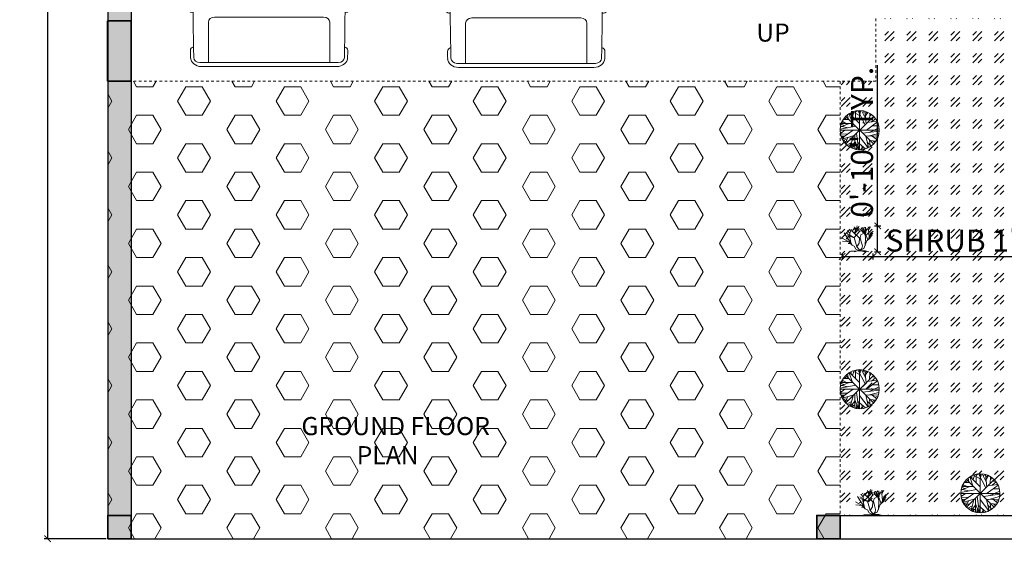
# Model space of a CAD drawing. Units: inches. Extents: x 3799 to 20199, y 1682 to 8087.
# Tile 6 of 30: x 10985 to 11366, y 2123 to 2325. Entities that reach past the tile are written whole.
import ezdxf

# ---------------------------------------------------------------- set-up
doc = ezdxf.new("R2010")
doc.units = ezdxf.units.IN
doc.linetypes.add('JIS_02_1.0', pattern=[2, 1, -1])
for name, color, linetype, lineweight in [('A-ANNO-DIMS', 2, 'Continuous', 18), ('A-ANNO-SYMB', 3, 'Continuous', 18), ('A-ANNO-TITL', 7, 'Continuous', 25), ('A-COLS', 251, 'Continuous', 35), ('A-SITE-OVHD', 8, 'JIS_02_1.0', 18), ('A-SITE-VEHC', 8, 'Continuous', 13), ('A-WALL-PATT', 252, 'Continuous', 13), ('C-PROP', 7, 'Continuous', 25), ('L-PAVE', 253, 'Continuous', 13), ('L-PLNT', 94, 'Continuous', 13), ('L-PLNT-PATT', 94, 'Continuous', 13)]:
    doc.layers.add(name, color=color, linetype=linetype, lineweight=lineweight)
doc.styles.get("Standard").update_dxf_attribs({"font": 'arial.ttf'})
doc.dimstyles.new('ISO-25', dxfattribs={"dimtxt": 8.5, "dimasz": 2.5, "dimexe": 1.25, "dimexo": 0.625, "dimtad": 1, "dimdec": 0, "dimlunit": 3, "dimtxsty": 'Standard', "dimblk": 'ARCHTICK', "dimcen": 2.5, "dimadec": 0, "dimazin": 0, "dimtfac": 1, "dimtdec": 0, "dimtmove": 0, "dimatfit": 3, "dimfxl": 1, "dimarcsym": 0})

# ---------------------------------------------------------------- blocks, each defined once
blk = doc.blocks.new('Shrub - elevation')
for p, q in [((-16.8, 16.32), (-18.72, 18.72)), ((-14.88, 18.24), (-17.76, 19.2)), ((-16.8, 16.32), (-15.36, 19.68)), ((-14.88, 18.24), (-12.96, 20.64)), ((-8.16, 12), (-14.88, 18.24)), ((-13.325, 16.724), (-11.433, 18.289)), ((-12.96, 12.48), (-8.16, 17.76)), ((-12.471, 19.775), (-12.898, 22.044)), ((-11.677, 19.071), (-12.471, 19.775)), ((-11.28, 19.619), (-12.104, 21.184)), ((-12.043, 15.628), (-11.921, 18.836)), ((-11.982, 16.802), (-10.579, 18.054)), ((-11.921, 18.836), (-10.64, 20.401)), ((-11.433, 18.289), (-10.457, 22.749)), ((-10.579, 18.054), (-9.846, 19.697)), ((-8.16, 17.76), (-10.56, 21.6)), ((-9.48, 19.775), (-8.992, 22.592)), ((-7.2, 19.68), (-8.64, 20.16)), ((-8.16, 17.76), (-5.28, 19.2)), ((-7.2, 19.68), (-6.24, 21.12)), ((-4.8, 16.32), (-7.2, 19.68)), ((-5.086, 17.741), (-5.513, 21.34)), ((-5.28, 19.2), (-3.84, 21.6)), ((-3.377, 15.315), (-5.086, 17.819)), ((-2.88, 12.96), (-4.32, 19.68)), ((-3.84, 16.8), (-0.96, 20.64)), ((-3.377, 18.602), (-2.888, 21.575)), ((-2.766, 16.802), (-3.377, 18.602)), ((-2.88, 15.84), (-2.4, 20.16)), ((-0.508, 21.888), (-0.081, 20.558)), ((-0.203, 19.149), (0.102, 21.34)), ((0.346, 13.203), (-0.203, 19.149)), ((-0.142, 19.384), (0.59, 20.401)), ((-0.02, 20.01), (0.896, 21.105)), ((0.041, 20.714), (1.384, 22.044)), ((0.102, 21.34), (0.835, 21.888)), ((1.323, 16.254), (3.642, 18.289)), ((-17.76, 8.64), (-23.663, 11.961)), ((-17.76, 8.64), (-23.128, 9.222)), ((-18.24, 11.04), (-21.755, 16.655)), ((-18.24, 11.04), (-20.16, 11.52)), ((-12.96, 12.48), (-19.68, 16.32)), ((-13.92, 12.48), (-19.2, 14.88)), ((-15.84, 8.16), (-18.24, 11.04)), ((-16.8, 12.48), (-17.76, 12.96)), ((-16.8, 12.48), (-16.8, 16.32)), ((-15.84, 8.16), (-16.8, 12.48)), ((-12.96, 12.48), (-13.92, 12.48)), ((-10.56, 4.32), (-12.96, 12.48)), ((-8.64, 7.68), (-8.16, 12)), ((-7.68, 12.48), (-7.2, 14.88)), ((-6.72, 8.64), (-7.68, 12.48)), ((-7.2, 14.88), (-3.84, 16.8)), ((-4.32, 2.88), (-1.92, 9.6)), ((-3.36, 5.28), (-2.88, 12.96)), ((-0.96, 10.56), (-2.88, 15.84)), ((-1.92, 9.6), (0.96, 12)), ((-0.48, 10.8), (0.346, 13.203)), ((0.346, 13.203), (1.323, 16.254)), ((0.96, 12), (1.44, 15.36)), ((0.96, 12), (2.88, 14.88)), ((1.44, 15.36), (2.88, 17.28)), ((1.92, 13.44), (2.4, 15.36)), ((2.4, 15.36), (3.36, 16.32)), ((-16.32, 7.2), (-18.24, 7.2)), ((-14.88, 5.76), (-17.76, 8.64)), ((-15.84, 0.48), (-17.76, 0)), ((-14.88, 5.76), (-15.84, 8.16)), ((-13.44, 0.48), (-15.84, 0.48)), ((-12.96, 4.8), (-14.88, 5.76)), ((-9.6, 0.96), (-13.44, 0.48)), ((-11.52, 2.4), (-12.96, 4.8)), ((-9.6, 0.96), (-12.96, 0)), ((-8.64, 0.96), (-11.52, 2.4)), ((-10.56, 4.32), (-8.64, 7.68)), ((-8.64, 1.92), (-10.56, 4.32)), ((-9.6, 0.96), (-7.68, 0.96)), ((-8.64, 0.96), (-4.32, 2.88)), ((-8.64, 0.96), (-6.24, 2.88)), ((-8.64, 0.96), (-8.64, 1.92)), ((-8.64, 0.96), (-2.88, 0.96)), ((-7.68, 0.96), (-6.24, 0.48)), ((-5.76, 5.28), (-6.72, 8.64)), ((-6.24, 2.88), (-5.76, 5.28)), ((-6.24, 0.48), (-3.36, 0)), ((-2.88, 0.96), (0, 0))]:
    blk.add_line(p, q)
blk = doc.blocks.new('Tree - deciduous plan')
for p, q in [((-49.8627, 32.8214), (-32.7853, 32.8214)), ((-45.8134, 38.2383), (-40.5318, 33.0471)), ((-43.8768, 36.4326), (-44.405, 40.2696)), ((42, 42), (-42, -42)), ((42, -42), (-42, 42)), ((-40.1797, 44.558), (-36.4825, 43.2038)), ((-37.0107, 47.0408), (-35.25, 35.5298)), ((-32.6092, 50.4264), (-23.2782, 23.5674)), ((-31.2008, 51.1035), (-0.2149, 20.1818)), ((-26.4472, 46.5894), (-26.2712, 53.8116)), ((-22.0458, 42.0753), (-16.5881, 57.6486)), ((-21.1656, 55.8436), (-0.0388, 45.0094)), ((-12.5388, 54.9406), (-7.9613, 59.4546)), ((-12.3627, 32.1443), (-12.5388, 58.7776)), ((-5.3205, 59.6806), (16.5105, 16.7963)), ((2.426, 54.9406), (-1.4472, 59.9056)), ((0, 59.9996), (0, -60)), ((0.4894, 48.6208), (3.6584, 59.6806)), ((18.2711, 35.5298), (5.419, 59.6806)), ((9.8203, 51.5549), (12.8133, 58.5516)), ((19.6795, 19.5047), (16.3344, 57.6486)), ((17.0387, 51.1035), (23.2006, 55.1666)), ((17.7429, 43.6552), (25.4894, 54.2636)), ((31.6513, 50.8778), (30.2429, 30.5643)), ((31.1232, 42.5267), (35.8767, 48.1693)), ((36.2288, 25.1474), (48.9049, 35.0784)), ((37.1091, 37.1098), (46.6161, 37.5612)), ((-59.7219, 2.8025), (-12.0106, 12.0565)), ((-32.2571, 20.6333), (-59.1937, 9.348)), ((-58.6656, 12.7336), (-35.9543, 7.5424)), ((-57.081, 17.9248), (-47.0458, 14.7649)), ((-56.0247, 20.859), (-20.8134, 20.859)), ((-54.7923, 24.4702), (-47.75, 21.0847)), ((-54.6162, -24.7335), (-20.2853, 0.0941)), ((-53.2078, 27.4044), (-40.1797, 20.859)), ((54.3626, 25.3731), (20.9119, 0.3198)), ((23.3767, 23.3417), (53.3063, 27.4044)), ((29.3626, -6.6771), (59.4682, 7.091)), ((38.5175, 13.4107), (58.2359, 13.6364)), ((-60, 0), (60, 0)), ((-59.7219, -4.8714), (-54.2641, -6.6771)), ((-45.2853, -0.1316), (-59.0177, -10.0627)), ((-58.4895, -12.3197), (-36.4825, -11.6426)), ((-57.081, -18.4138), (-45.2853, -17.9624)), ((-52.6797, -18.188), (-55.4966, -22.0251)), ((-53.2078, -27.442), (-16.7641, -16.6081)), ((-38.9472, -29.0219), (-51.4472, -30.6018)), ((-47.2219, -19.3166), (-50.2148, -26.3135)), ((-46.5177, -30.1504), (-49.5106, -33.536)), ((-35.9543, -22.4765), (-44.0529, -40.5329)), ((-19.9331, -20.2194), (-28.5599, -52.721)), ((-14.8275, -15.0282), (-14.6515, -57.6865)), ((-10.074, -10.0627), (-2.5036, -59.7178)), ((-0.0388, -19.0909), (25.8415, -53.8495)), ((9.2922, -9.1598), (59.6443, -2.8401)), ((18.6232, -18.6394), (26.7218, -53.3981)), ((18.7992, -18.6394), (57.3556, -17.2853)), ((26.3697, -18.4138), (58.9401, -9.8369)), ((30.419, -30.1504), (32.3556, -50.0125)), ((38.1654, -18.188), (52.426, -29.0219)), ((45.9119, -24.0564), (55.595, -22.2508)), ((-32.4331, -32.4075), (-48.1021, -35.5674)), ((-43.7008, -34.6645), (-46.6937, -37.373)), ((-24.6867, -37.8244), (-38.7712, -45.7241)), ((-26.2712, -43.9185), (-34.7219, -48.6583)), ((-14.6515, -36.2445), (-27.6797, -52.9467)), ((-14.6515, -47.3041), (-25.0388, -54.3009)), ((-21.5177, -45.4984), (-19.9331, -56.1065)), ((-14.6515, -32.1818), (-3.912, -59.4922)), ((-8.4895, -47.5298), (-11.4825, -58.5893)), ((-6.3768, -52.721), (-9.3698, -58.815)), ((-6.2008, -36.2445), (17.919, -57.0094)), ((8.4119, -53.1724), (3.8344, -59.4922)), ((5.9471, -46.6269), (10.5246, -58.5893)), ((22.8485, -36.4702), (35.3485, -48.4326)), ((24.7852, -44.8213), (23.0246, -54.978)), ((31.4753, -31.279), (49.6091, -33.3103)), ((41.5105, -32.6332), (46.088, -38.0501))]:
    blk.add_line(p, q)
blk.add_circle((0, 0), 60)
blk = doc.blocks.new('_ArchTick')
at = {"color": 0, "linetype": 'ByBlock', "const_width": 0.15}
blk.add_lwpolyline([(-0.5, -0.5), (0.5, 0.5)], dxfattribs=at)
blk = doc.blocks.new('*D77')
at = {"layer": 'A-ANNO-DIMS', "color": 0, "lineweight": -2, "transparency": 16777216}
for p, q in [((11018.23, 3204.07), (10994.27, 3204.07)), ((10995.52, 3204.07), (10995.52, 2124.07)), ((11018.23, 2124.07), (10994.27, 2124.07))]:
    blk.add_line(p, q, dxfattribs=at)
at = {"layer": 'Defpoints', "color": 0, "transparency": 16777216}
for p in [(11018.85, 3204.07), (10995.52, 2124.07), (11018.85, 2124.07)]:
    blk.add_point(p, dxfattribs=at)
at = {"layer": 'A-ANNO-DIMS', "color": 0, "lineweight": -2, "transparency": 16777216, "xscale": 2.5, "yscale": 2.5, "zscale": 2.5}
for p, rotation in [((10995.52, 3204.07), 90), ((10995.52, 2124.07), 270)]:
    blk.add_blockref('_ArchTick', p, dxfattribs=dict(at, rotation=rotation))
at = {"layer": 'A-ANNO-DIMS', "color": 0, "transparency": 16777216, "insert": (10990.56, 2664.07), "char_height": 8.5, "attachment_point": 5, "rotation": 90}
blk.add_mtext("90'", dxfattribs=at)
blk = doc.blocks.new('*U92')
for p, q in [((46.55, 38.89), (22.35, 38.89)), ((136.7, 38.89), (160.9, 38.89)), ((21.1, 37.41), (21.1, 36.83)), ((47.8, 37.39), (47.8, 37.41)), ((87.99, 31.87), (74.76, 35.92)), ((134.31, 35.6), (119.29, 31.78)), ((135.45, 37.07), (135.45, 37.41)), ((162.15, 37.41), (162.15, 36.77)), ((186.47, -33.5), (186.47, 33.5)), ((70.03, 31.54), (86.41, 29.35)), ((138.42, 29.35), (157.25, 29.35)), ((186.47, 29.35), (167.01, 29.35)), ((188.4, -32.76), (188.4, 32.76)), ((164.52, 26.39), (164.52, -26.39)), ((32.27, 11.63), (36.13, 17.17)), ((36.13, 17.17), (50.94, 17.17)), ((32.12, 9.51), (32.12, 11.15)), ((58.92, -10.77), (58.92, 10.77)), ((66.55, -10.53), (66.55, 10.53)), ((186.47, -10.53), (186.47, 10.53)), ((3.27, 6.13), (0.1, 0.41)), ((29.77, 9.51), (51.68, 9.51)), ((82.74, 8.5), (82.74, -8.5)), ((0, 0), (51.68, 0)), ((0.1, -0.41), (3.27, -6.13)), ((29.77, -9.51), (51.68, -9.51)), ((32.12, -9.51), (32.12, -11.15)), ((32.27, -11.63), (36.13, -17.17)), ((36.13, -17.17), (50.94, -17.17)), ((86.41, -29.35), (70.03, -31.54)), ((87.99, -31.87), (74.76, -35.92)), ((134.31, -35.6), (119.29, -31.78)), ((157.25, -29.35), (138.42, -29.35)), ((167.01, -29.35), (186.47, -29.35)), ((21.1, -37.41), (21.1, -36.83)), ((47.8, -37.39), (47.8, -37.41)), ((135.45, -37.07), (135.45, -37.41)), ((162.15, -37.41), (162.15, -36.77)), ((46.55, -38.89), (22.35, -38.89)), ((136.7, -38.89), (160.9, -38.89))]:
    blk.add_line(p, q)
for centre, major_axis, ratio, start_param, end_param in [((22.35, 37.41), (0, -1.48), 0.842304, 3.141593, 4.712389), ((46.55, 37.41), (0, 1.48), 0.842304, -1.570796, 0), ((136.7, 37.41), (0, -1.48), 0.842304, 3.141593, 4.712389), ((160.9, 37.41), (0, 1.48), 0.842304, -1.570796, 0), ((266.03, -27.52), (0, 313.31), 0.842304, 1.367076, 1.39176), ((41.19, -490.86), (0, 528.23), 0.842304, 0.00281, 0.075598), ((64.48, -10555.62), (0, 10593.03), 0.842304, -0.013397, 0.002797), ((64.48, -10555.62), (0, -10591.55), 0.842304, 3.133765, 3.140441), ((180.63, 35.84), (0, 2.22), 0.842304, -0.013017, 1.249894), ((64.48, -10556.36), (0, 10595.31), 0.842304, -0.013397, -0.013017), ((183.98, 33.5), (0, -2.96), 0.842304, 1.570796, 3.128196), ((183.98, 32.76), (0, -5.25), 0.842304, 1.570796, 3.128196), ((37.47, -593.96), (0, -623.33), 0.842304, 3.096046, 3.200911), ((134.4, 5.39), (0, -89.78), 0.842304, 4.449482, 4.652344), ((135.29, 5.39), (0, 81.77), 0.842304, 1.245306, 1.50788), ((149.6, 2.8), (0, -79.58), 0.842304, 4.372215, 4.640744), ((95.79, -3666.35), (0, -3698.24), 0.842304, 3.134049, 3.144098), ((17.08, 0), (0, 147.02), 0.842304, 4.511394, 4.913384), ((35.91, 0), (0, 147.02), 0.842304, 4.511394, 4.913384), ((167.01, 26.39), (0, 2.96), 0.842304, 0, 1.570796), ((259.18, -27.52), (0, -305.3), 0.842304, 4.528606, 4.561838), ((-204.49, 52.4), (0, -250.96), 0.842304, 1.385369, 1.434372), ((13.04, 17.01), (0, 27.42), 0.842304, 4.435146, 4.718221), ((14.2, 17.01), (0, 27.42), 0.842304, 4.435146, 4.718221), ((50.79, 13.34), (6.34, -0.36), 0.603834, -1.395552, 1.581315), ((32.75, 11.15), (0, 0.74), 0.842304, 0.879714, 1.570796), ((29.77, -46.66), (0, 56.17), 0.842304, 0, 0.590319), ((0.62, 0), (0, -0.74), 0.842304, 4.131459, 5.293319), ((29.77, 46.66), (0, 56.17), 0.842304, 2.551274, 3.141593), ((-204.49, -52.4), (0, 250.96), 0.842304, -1.434372, -1.385369), ((13.04, -17.01), (0, -27.42), 0.842304, 1.564964, 1.848039), ((14.2, -17.01), (0, -27.42), 0.842304, 1.564964, 1.848039), ((149.6, -2.8), (0, -79.58), 0.842304, -1.499151, -1.230623), ((32.75, -11.15), (0, -0.74), 0.842304, 4.712389, 5.403472), ((134.4, -5.39), (0, -89.78), 0.842304, -1.510751, -1.307889), ((135.29, -5.39), (0, -81.77), 0.842304, -1.50788, -1.245306), ((259.18, 27.52), (0, 305.3), 0.842304, 1.721348, 1.754579), ((266.03, 27.52), (0, 313.31), 0.842304, 1.749832, 1.774517), ((37.47, 593.96), (0, -623.33), 0.842304, -0.059319, 0.045547), ((167.01, -26.39), (0, -2.96), 0.842304, 4.712389, 6.283185), ((95.79, 3666.35), (0, -3698.24), 0.842304, -0.002505, 0.007544), ((183.98, -32.76), (0, -5.25), 0.842304, 0.013397, 1.570796), ((41.19, 490.86), (0, -528.23), 0.842304, -0.075598, -0.00281), ((22.35, -37.41), (0, 1.48), 0.842304, 1.570796, 3.141593), ((64.48, 10555.62), (0, 10593.03), 0.842304, 3.138796, 3.15499), ((46.55, -37.41), (0, -1.48), 0.842304, 0, 1.570796), ((64.48, 10555.62), (0, -10591.55), 0.842304, 0.001152, 0.007828), ((136.7, -37.41), (0, -1.48), 0.842304, -1.570796, 0), ((160.9, -37.41), (0, 1.48), 0.842304, 3.141593, 4.712389), ((180.63, -35.84), (0, -2.22), 0.842304, -1.249894, 0.013017), ((64.48, 10556.36), (0, 10595.31), 0.842304, 3.15461, 3.15499), ((183.98, -33.5), (0, 2.96), 0.842304, 3.15499, 4.712389)]:
    blk.add_ellipse(centre, major_axis=major_axis, ratio=ratio, start_param=start_param, end_param=end_param)
at = {"extrusion": (0, 0, -1)}
blk.add_ellipse((50.79, -13.34), major_axis=(6.34, 0.36), ratio=0.603834, start_param=-1.395552, end_param=1.581315, dxfattribs=at)
blk = doc.blocks.new('*D300')
at = {"layer": 'A-ANNO-DIMS', "color": 0, "lineweight": -2, "transparency": 16777216}
for p, q in [((11302.78, 2234.32), (11302.78, 2231.9)), ((11302.78, 2233.15), (11314.75, 2233.15)), ((11314.75, 2234.32), (11314.75, 2231.9)), ((11314.75, 2233.15), (11415.14, 2233.15))]:
    blk.add_line(p, q, dxfattribs=at)
at = {"layer": 'Defpoints', "color": 0, "transparency": 16777216}
for p in [(11302.78, 2234.95), (11314.75, 2234.95), (11314.75, 2233.15)]:
    blk.add_point(p, dxfattribs=at)
at = {"layer": 'A-ANNO-DIMS', "color": 0, "lineweight": -2, "transparency": 16777216, "xscale": 2.5, "yscale": 2.5, "zscale": 2.5, "rotation": 180}
blk.add_blockref('_ArchTick', (11302.78, 2233.15), dxfattribs=at)
at = {"layer": 'A-ANNO-DIMS', "color": 0, "lineweight": -2, "transparency": 16777216, "xscale": 2.5, "yscale": 2.5, "zscale": 2.5}
blk.add_blockref('_ArchTick', (11314.75, 2233.15), dxfattribs=at)
at = {"layer": 'A-ANNO-DIMS', "color": 0, "transparency": 16777216, "insert": (11366.2, 2238.17), "char_height": 8.5, "attachment_point": 5}
blk.add_mtext('SHRUB 1\'-0" TYP.', dxfattribs=at)
blk = doc.blocks.new('*D301')
at = {"layer": 'A-ANNO-DIMS', "color": 0, "lineweight": -2, "transparency": 16777216}
for p, q in [((11316.55, 2244.93), (11316.55, 2307.09)), ((11315.38, 2244.93), (11317.8, 2244.93)), ((11316.55, 2234.95), (11316.55, 2244.93)), ((11315.38, 2234.95), (11317.8, 2234.95))]:
    blk.add_line(p, q, dxfattribs=at)
at = {"layer": 'Defpoints', "color": 0, "transparency": 16777216}
for p in [(11314.75, 2244.93), (11316.55, 2244.93), (11314.75, 2234.95)]:
    blk.add_point(p, dxfattribs=at)
at = {"layer": 'A-ANNO-DIMS', "color": 0, "lineweight": -2, "transparency": 16777216, "xscale": 2.5, "yscale": 2.5, "zscale": 2.5}
for p, rotation in [((11316.55, 2244.93), 90), ((11316.55, 2234.95), 270)]:
    blk.add_blockref('_ArchTick', p, dxfattribs=dict(at, rotation=rotation))
at = {"layer": 'A-ANNO-DIMS', "color": 0, "transparency": 16777216, "insert": (11311.58, 2277.26), "char_height": 8.5, "attachment_point": 5, "rotation": 90}
blk.add_mtext('0\'-10" TYP.', dxfattribs=at)

msp = doc.modelspace()

# ---------------------------------------------------------------- hatches: boundary and pattern name
at = {"layer": 'A-COLS'}
h = msp.add_hatch(color=256, dxfattribs=at)
h.dxf.hatch_style = 1
h.set_gradient(color1=(0, 0, 255), color2=(122, 175, 223))
h.paths.add_polyline_path([(11302.02, 2133.07), (11293.02, 2133.07), (11293.02, 2124.07), (11302.02, 2124.07)])
h.paths.add_polyline_path([(11027.85, 2133.07), (11018.85, 2133.07), (11018.85, 2124.07), (11027.85, 2124.07)])
h.paths.add_polyline_path([(11027.85, 2324.17), (11018.85, 2324.17), (11018.85, 2300.82), (11027.85, 2300.82)])
h.paths.add_polyline_path([(11027.85, 2493.31), (11018.85, 2493.31), (11018.85, 2469.95), (11027.85, 2469.95)])
at = {"layer": 'A-WALL-PATT'}
h = msp.add_hatch(color=256, dxfattribs=at)
h.dxf.hatch_style = 1
h.paths.add_polyline_path([(11027.85, 2469.95), (11018.85, 2469.95), (11018.85, 2324.17), (11027.85, 2324.17)])
h.paths.add_polyline_path([(11027.85, 2300.82), (11018.85, 2300.82), (11018.85, 2133.07), (11027.85, 2133.07)])
at = {"layer": 'L-PAVE'}
h = msp.add_hatch(dxfattribs=at)
h.set_pattern_fill('HEX', color=256, scale=2)
h.paths.add_polyline_path([(11302.02, 2300.82), (11018.85, 2300.82), (11018.85, 2124.07), (11302.02, 2124.07)])
h.paths.add_polyline_path([(11091.95, 2151.09), (11148.17, 2151.09), (11148.17, 2161.6), (11091.95, 2161.6)], flags=24)
h.paths.add_polyline_path([(11091.89, 2162.16), (11175.38, 2162.16), (11175.38, 2173.03), (11091.89, 2173.02)], flags=24)
at = {"layer": 'L-PLNT-PATT'}
h = msp.add_hatch(dxfattribs=at)
h.set_pattern_fill('GOST_GLASS', color=256)
h.paths.add_polyline_path([(11609.85, 2325.07), (11549.85, 2325.07), (11315.85, 2325.07), (11315.85, 2300.82), (11302.02, 2300.82), (11302.02, 2133.07), (11609.85, 2133.07)])
h.paths.add_polyline_path([(11496.55, 2144.31), (11496.62, 2144.39), (11496.58, 2144.52)], flags=16)
h.paths.add_polyline_path([(11491.91, 2145.12), (11493.01, 2143.36), (11494.28, 2143.99), (11494.28, 2144.01), (11494.36, 2143.39), (11494.73, 2142.84), (11494.91, 2142.94), (11495.46, 2143.67), (11495.33, 2142.52), (11496.19, 2140.15), (11495.75, 2139.78), (11494.7, 2136.83), (11492.98, 2136.07), (11493.22, 2135.99), (11492.8, 2135.99), (11491.54, 2136.62), (11490.91, 2137.68), (11490.07, 2138.1), (11489.64, 2139.15), (11489.22, 2141.04), (11489.22, 2142.73), (11489.64, 2143.71), (11490.07, 2143.57), (11491.02, 2144.77), (11491.12, 2144.24), (11491.46, 2143.95), (11491.73, 2144.28)], flags=16)
h.paths.add_polyline_path([(11491.31, 2142.42), (11493.01, 2140.83), (11492.8, 2138.94), (11491.96, 2137.47), (11490.91, 2141.04), (11491.77, 2141.99), (11490.77, 2142.92), (11491.35, 2143.4)], flags=0)
h.paths.add_polyline_path([(11455.55, 2140.87), (11453.52, 2140.87), (11451.69, 2140.04), (11455.54, 2140.52, 0.011687)], flags=16)
h.paths.add_polyline_path([(11451.82, 2137.03), (11451.82, 2136.94), (11451.92, 2136.93)], flags=16)
h.paths.add_polyline_path([(11447.97, 2140.87), (11447.97, 2135.62), (11447.21, 2136.28), (11446.7, 2139.6), (11446.1, 2139), (11446.11, 2136.84), (11446.26, 2136.47), (11446.11, 2136.28), (11446.12, 2134.9), (11445.36, 2134.39), (11445.25, 2135.18), (11446.11, 2136.28), (11446.1, 2138.85), (11445.88, 2138.78), (11443.88, 2136.78), (11442.77, 2136.56), (11443.44, 2138.06), (11441.62, 2137.52), (11442.08, 2138.6), (11442.26, 2138.61), (11442, 2138.42), (11441.62, 2137.52), (11445.88, 2138.78), (11447.97, 2140.87), (11447.97, 2143.39), (11445.18, 2146.18), (11445.72, 2147.71), (11447.97, 2146.55), (11447.97, 2148.2), (11448.27, 2147.82), (11448.02, 2146.98), (11450.07, 2142.97)], flags=16)
h.paths.add_polyline_path([(11551.41, 2140.65, -1), (11536.26, 2140.65, -1)])
h.paths.add_polyline_path([(11547.68, 2136.8), (11547.69, 2136.71), (11547.78, 2136.7)], flags=16)
h.paths.add_polyline_path([(11541.05, 2145.95), (11541.58, 2147.48), (11542.26, 2147.14), (11542.27, 2144.73)], flags=16)
h.paths.add_polyline_path([(11541.96, 2138.78), (11541.97, 2136.62), (11542.12, 2136.24), (11541.97, 2136.06), (11541.98, 2134.67), (11541.23, 2134.17), (11541.11, 2134.95), (11541.97, 2136.06), (11541.96, 2138.62), (11541.74, 2138.56), (11539.74, 2136.56), (11538.63, 2136.33), (11539.3, 2137.83), (11537.48, 2137.29), (11537.94, 2138.37), (11538.12, 2138.38), (11541.25, 2140.65), (11543.83, 2140.65)], flags=16)
h.paths.add_polyline_path([(11584.29, 2268.01), (11584.1, 2268.75), (11584.25, 2269.39), (11584.02, 2270.08), (11583.56, 2270.33), (11584.06, 2270.63), (11584.18, 2271.22), (11584.1, 2271.81), (11584.48, 2272.21), (11584.83, 2272.85), (11584.45, 2273.49), (11583.87, 2273.79), (11584.72, 2273.79), (11585.41, 2273.89), (11585.79, 2274.33), (11585.79, 2274.73), (11586.3, 2275.17), (11587.03, 2275.22), (11587.76, 2275.66), (11588.26, 2275.62), (11588.72, 2275.91), (11589.22, 2275.66), (11589.53, 2276.8), (11589.69, 2275.91), (11590.23, 2275.81), (11590.92, 2276.11), (11591.46, 2276.26), (11592.73, 2275.22), (11593.19, 2274.92), (11593.58, 2275.12), (11594.35, 2274.87), (11594.31, 2274.38), (11594.43, 2274.03), (11595.08, 2273.34), (11595.47, 2272.9), (11595.54, 2271.76), (11595.89, 2271.47), (11596.85, 2271.47), (11597.55, 2271.52), (11596.78, 2271.22), (11596.08, 2270.87), (11595.93, 2270.43), (11596.04, 2269.79), (11595.85, 2269.58), (11596.25, 2269.39), (11596.63, 2270.81), (11596.82, 2269.7), (11597.5, 2269.57), (11598.36, 2269.94), (11599.04, 2270.13), (11600.63, 2268.83), (11601.21, 2268.46), (11601.77, 2268.75), (11601.65, 2268.95), (11601.29, 2269.14), (11601.82, 2269.14), (11602.25, 2269.2), (11602.49, 2269.48), (11602.49, 2269.72), (11602.81, 2270), (11603.26, 2270.03), (11603.72, 2270.31), (11604.04, 2270.28), (11604.32, 2270.46), (11604.64, 2270.31), (11604.83, 2271.02), (11604.93, 2270.46), (11605.26, 2270.4), (11605.7, 2270.59), (11606.03, 2270.68), (11606.83, 2270.03), (11607.12, 2269.85), (11607.36, 2269.97), (11607.84, 2269.82), (11607.82, 2269.51), (11607.89, 2269.29), (11608.3, 2268.86), (11608.54, 2268.58), (11608.59, 2267.87), (11608.8, 2267.68), (11609.4, 2267.68), (11609.84, 2267.72), (11609.36, 2267.53), (11608.92, 2267.31), (11608.83, 2267.04), (11608.9, 2266.64), (11608.73, 2266.45), (11608.63, 2265.68), (11608.75, 2265.52), (11608.66, 2265.46), (11608.44, 2265.04), (11608.03, 2264.97), (11608.39, 2264.54), (11607.96, 2264.63), (11607.84, 2264.57), (11607.82, 2264.32), (11607.45, 2263.98), (11607.26, 2263.7), (11606.85, 2263.64), (11606.54, 2263.39), (11606.01, 2263.24), (11605.65, 2263.27), (11605.31, 2263.15), (11605.21, 2263.02), (11605.12, 2262.28), (11604.9, 2263.02), (11604.71, 2263.08), (11604.63, 2262.84), (11604.77, 2262.04), (11604.43, 2261.67), (11604.24, 2260.13), (11604.48, 2259.82), (11604.29, 2259.69), (11604, 2259.14), (11603.76, 2258.83), (11603.04, 2258.71), (11603.76, 2257.84), (11602.89, 2258.03), (11602.65, 2257.9), (11602.6, 2257.41), (11601.88, 2256.73), (11601.49, 2256.17), (11600.68, 2256.05), (11600.05, 2255.56), (11598.99, 2255.25), (11598.27, 2255.31), (11597.59, 2255.06), (11597.4, 2254.82), (11597.21, 2253.33), (11596.77, 2254.82), (11595.19, 2255.25), (11594.51, 2255.31), (11593.79, 2255.87), (11593.21, 2256.48), (11592.73, 2256.61), (11592.1, 2256.17), (11591.48, 2255.56), (11591.81, 2256.36), (11591.91, 2257.47), (11591.53, 2257.96), (11590.75, 2258.34), (11590.75, 2258.95), (11590.61, 2259.45), (11590.08, 2259.82), (11589.84, 2260.74), (11590.03, 2261.55), (11589.74, 2262.41), (11589.17, 2262.72), (11589.79, 2263.09), (11589.84, 2263.34), (11589.65, 2264.01), (11588.38, 2264.35), (11587.84, 2264.4), (11587.26, 2264.85), (11586.8, 2265.34), (11586.41, 2265.44), (11585.91, 2265.09), (11585.41, 2264.6), (11585.68, 2265.24), (11585.76, 2266.13), (11585.45, 2266.53), (11584.83, 2266.82), (11584.83, 2267.32), (11584.72, 2267.71)], flags=16)
h.paths.add_polyline_path([(11589.76, 2270.08), (11589.88, 2270.23), (11589.99, 2270.08)], flags=0)
h.paths.add_polyline_path([(11596.92, 2262.41), (11597.06, 2262.6), (11597.21, 2262.41)], flags=0)
h.paths.add_polyline_path([(11607.36, 2210.31), (11607.43, 2210.39), (11607.39, 2210.52)], flags=16)
h.paths.add_polyline_path([(11600.87, 2204.1), (11600.45, 2205.15), (11600.03, 2207.04), (11600.03, 2208.73), (11600.45, 2209.71), (11600.87, 2209.57), (11601.83, 2210.77), (11601.93, 2210.24), (11602.27, 2209.95), (11602.54, 2210.28), (11602.72, 2211.12), (11603.82, 2209.36), (11605.09, 2209.99), (11605.09, 2210), (11605.17, 2209.39), (11605.54, 2208.84), (11605.72, 2208.94), (11606.27, 2209.67), (11606.14, 2208.52), (11607, 2206.15), (11606.56, 2205.78), (11605.51, 2202.83), (11603.79, 2202.07), (11604.03, 2201.99), (11603.61, 2201.99), (11602.35, 2202.62), (11601.72, 2203.68)], flags=16)
h.paths.add_polyline_path([(11601.72, 2207.04), (11602.58, 2207.99), (11601.57, 2208.92), (11602.16, 2209.4), (11602.12, 2208.42), (11603.82, 2206.83), (11603.61, 2204.94), (11602.77, 2203.47)], flags=0)
h.paths.add_polyline_path([(11399.57, 2144.02), (11399.64, 2144.1), (11399.6, 2144.23)], flags=16)
h.paths.add_polyline_path([(11398.77, 2139.49), (11397.71, 2136.54), (11396, 2135.78), (11396.24, 2135.7), (11395.82, 2135.7), (11394.55, 2136.33), (11393.92, 2137.38), (11393.08, 2137.81), (11392.66, 2138.86), (11392.24, 2140.75), (11392.24, 2142.44), (11392.66, 2143.42), (11393.08, 2143.28), (11394.04, 2144.48), (11394.14, 2143.95), (11394.47, 2143.66), (11394.74, 2143.99), (11394.93, 2144.83), (11396.03, 2143.07), (11397.29, 2143.7), (11397.3, 2143.71), (11397.37, 2143.1), (11397.75, 2142.55), (11397.92, 2142.65), (11398.47, 2143.38), (11398.34, 2142.23), (11399.21, 2139.86)], flags=16)
h.paths.add_polyline_path([(11609.04, 2180.55, -1), (11593.89, 2180.55, -1)], flags=16)
h.paths.add_polyline_path([(11605.31, 2176.71), (11605.32, 2176.61), (11605.41, 2176.6)], flags=0)
h.paths.add_polyline_path([(11601.47, 2180.55), (11601.47, 2183.07), (11598.68, 2185.85), (11599.22, 2187.38), (11601.47, 2186.23), (11601.47, 2187.88), (11601.76, 2187.5), (11601.52, 2186.66), (11603.57, 2182.65), (11601.47, 2180.55), (11601.47, 2175.3), (11600.7, 2175.96), (11600.2, 2179.28), (11599.6, 2178.68), (11599.61, 2176.52), (11599.75, 2176.15), (11599.61, 2175.96), (11599.61, 2174.57), (11598.86, 2174.07), (11598.74, 2174.85), (11599.61, 2175.96), (11599.6, 2178.53), (11599.38, 2178.46), (11597.38, 2176.46), (11596.27, 2176.23), (11596.94, 2177.74), (11595.11, 2177.19), (11595.58, 2178.28), (11595.76, 2178.28), (11598.89, 2180.55)], flags=0)
h.paths.add_polyline_path([(11394.33, 2142.12), (11396.03, 2140.54), (11395.82, 2138.65), (11394.98, 2137.17), (11393.92, 2140.75), (11394.78, 2141.7), (11393.78, 2142.63), (11394.36, 2143.11)], flags=0)
h.paths.add_polyline_path([(11604.97, 2266.82), (11605.05, 2266.91), (11605.12, 2266.82)], flags=0)
h.paths.add_polyline_path([(11593.36, 2312.93, -1), (11608.51, 2312.93, -1)], flags=16)
h.paths.add_polyline_path([(11604.78, 2309.09), (11604.79, 2309), (11604.88, 2308.99)], flags=0)
h.paths.add_polyline_path([(11596.4, 2310.12), (11594.58, 2309.58), (11595.04, 2310.66), (11595.22, 2310.66), (11598.35, 2312.93), (11600.93, 2312.93), (11600.93, 2315.45), (11598.15, 2318.23), (11598.68, 2319.77), (11600.93, 2318.61), (11600.93, 2320.26), (11601.23, 2319.88), (11600.99, 2319.04), (11603.03, 2315.03), (11600.93, 2312.93), (11600.93, 2307.68), (11600.17, 2308.34), (11599.66, 2311.66), (11599.06, 2311.06), (11599.07, 2308.9), (11599.22, 2308.53), (11599.07, 2308.34), (11599.08, 2306.96), (11598.33, 2306.45), (11598.21, 2307.24), (11599.07, 2308.34), (11599.06, 2310.91), (11598.84, 2310.84), (11596.84, 2308.84), (11595.73, 2308.62)], flags=0)
h.paths.add_polyline_path([(11605.66, 2145.72), (11605.73, 2145.8), (11605.69, 2145.93)], flags=16)
h.paths.add_polyline_path([(11598.75, 2140.56), (11598.33, 2142.46), (11598.33, 2144.14), (11598.75, 2145.12), (11599.17, 2144.98), (11600.13, 2146.18), (11600.23, 2145.66), (11600.56, 2145.36), (11600.83, 2145.69), (11601.02, 2146.53), (11602.12, 2144.77), (11603.38, 2145.4), (11603.39, 2145.42), (11603.46, 2144.81), (11603.84, 2144.25), (11604.02, 2144.35), (11604.56, 2145.08), (11604.44, 2143.93), (11605.3, 2141.56), (11604.86, 2141.19), (11603.8, 2138.25), (11602.09, 2137.48), (11602.33, 2137.4), (11601.91, 2137.4), (11600.65, 2138.04), (11600.01, 2139.09), (11599.17, 2139.51)], flags=16)
h.paths.add_polyline_path([(11600.01, 2142.46), (11600.87, 2143.4), (11599.87, 2144.33), (11600.45, 2144.81), (11600.42, 2143.83), (11602.12, 2142.25), (11601.91, 2140.35), (11601.07, 2138.88)], flags=0)
h.paths.add_polyline_path([(11363.83, 2141.59, -1), (11348.68, 2141.59, -1)], flags=0)
h.paths.add_polyline_path([(11360.1, 2137.75), (11360.11, 2137.66), (11360.2, 2137.65)], flags=0)
h.paths.add_polyline_path([(11356.26, 2141.59), (11356.26, 2136.34), (11355.49, 2137), (11354.98, 2140.32), (11354.38, 2139.72), (11354.39, 2137.56), (11354.54, 2137.19), (11354.39, 2137), (11354.4, 2135.62), (11353.65, 2135.11), (11353.53, 2135.9), (11354.39, 2137), (11354.38, 2139.57), (11354.17, 2139.5), (11352.16, 2137.5), (11351.05, 2137.28), (11351.73, 2138.78), (11349.9, 2138.24), (11350.36, 2139.32), (11350.54, 2139.33), (11353.68, 2141.59), (11356.26, 2141.59), (11356.26, 2144.11), (11353.47, 2146.9), (11354.01, 2148.43), (11356.26, 2147.27), (11356.26, 2148.92), (11356.55, 2148.54), (11356.31, 2147.7), (11358.35, 2143.69)], flags=0)
h.paths.add_polyline_path([(11313.11, 2243.68), (11313.18, 2243.77), (11313.14, 2243.89)], flags=16)
h.paths.add_polyline_path([(11312.31, 2239.16), (11311.26, 2236.21), (11309.55, 2235.45), (11309.79, 2235.37), (11309.37, 2235.37), (11308.1, 2236), (11307.47, 2237.05), (11306.63, 2237.47), (11306.21, 2238.53), (11305.79, 2240.42), (11305.79, 2242.11), (11306.21, 2243.09), (11306.63, 2242.95), (11307.59, 2244.15), (11307.68, 2243.62), (11308.02, 2243.32), (11308.29, 2243.65), (11308.47, 2244.5), (11309.58, 2242.74), (11310.84, 2243.37), (11310.85, 2243.38), (11310.92, 2242.77), (11311.3, 2242.22), (11311.47, 2242.32), (11312.02, 2243.05), (11311.89, 2241.9), (11312.75, 2239.53)], flags=16)
h.paths.add_polyline_path([(11308.52, 2236.84), (11307.47, 2240.42), (11308.33, 2241.37), (11307.33, 2242.3), (11307.91, 2242.78), (11307.87, 2241.79), (11309.58, 2240.21), (11309.37, 2238.32)], flags=0)
h.paths.add_polyline_path([(11302.02, 2281.94, -1), (11317.17, 2281.94, -1)])
h.paths.add_polyline_path([(11313.44, 2278.1), (11313.44, 2278), (11313.54, 2277.99)], flags=16)
h.paths.add_polyline_path([(11309.59, 2276.69), (11308.83, 2277.35), (11308.32, 2280.67), (11307.72, 2280.07), (11307.73, 2277.91), (11307.88, 2277.54), (11307.73, 2277.35), (11307.74, 2275.96), (11306.98, 2275.46), (11306.87, 2276.24), (11307.73, 2277.35), (11307.72, 2279.92), (11307.5, 2279.85), (11305.5, 2277.85), (11304.39, 2277.63), (11305.06, 2279.13), (11303.24, 2278.58), (11303.7, 2279.67), (11303.88, 2279.67), (11303.62, 2279.49), (11303.24, 2278.58), (11307.5, 2279.85), (11309.59, 2281.94), (11309.59, 2284.46), (11306.8, 2287.24), (11307.34, 2288.77), (11309.59, 2287.62), (11309.59, 2289.27), (11309.89, 2288.89), (11309.64, 2288.05), (11311.69, 2284.04), (11309.59, 2281.94)], flags=16)
h.paths.add_polyline_path([(11317.17, 2181.83, -1), (11302.02, 2181.83, -1)])
h.paths.add_polyline_path([(11313.44, 2177.98), (11313.44, 2177.89), (11313.54, 2177.88)], flags=16)
h.paths.add_polyline_path([(11309.59, 2181.83), (11309.59, 2176.58), (11308.83, 2177.24), (11308.32, 2180.56), (11307.72, 2179.96), (11307.73, 2177.8), (11307.88, 2177.42), (11307.73, 2177.24), (11307.74, 2175.85), (11306.98, 2175.35), (11306.87, 2176.13), (11307.73, 2177.24), (11307.72, 2179.8), (11307.5, 2179.74), (11305.5, 2177.74), (11304.39, 2177.51), (11305.06, 2179.01), (11303.24, 2178.47), (11303.7, 2179.55), (11303.88, 2179.56), (11303.62, 2179.38), (11303.24, 2178.47), (11307.5, 2179.74), (11309.59, 2181.83), (11309.59, 2184.35), (11306.8, 2187.13), (11307.34, 2188.66), (11309.59, 2187.51), (11309.59, 2189.16), (11309.89, 2188.78), (11309.64, 2187.94), (11311.69, 2183.93)], flags=16)
h.paths.add_polyline_path([(11318.27, 2141.81), (11318.34, 2141.89), (11318.3, 2142.02)], flags=16)
h.paths.add_polyline_path([(11317.47, 2137.28), (11316.41, 2134.34), (11314.7, 2133.57), (11314.94, 2133.49), (11314.52, 2133.49), (11313.26, 2134.12), (11312.62, 2135.18), (11311.78, 2135.6), (11311.36, 2136.65), (11310.94, 2138.55), (11310.94, 2140.23), (11311.36, 2141.21), (11311.78, 2141.07), (11312.74, 2142.27), (11312.84, 2141.75), (11313.17, 2141.45), (11313.44, 2141.78), (11313.63, 2142.62), (11314.73, 2140.86), (11315.99, 2141.49), (11316, 2141.51), (11316.07, 2140.9), (11316.45, 2140.34), (11316.62, 2140.44), (11317.17, 2141.17), (11317.05, 2140.02), (11317.91, 2137.65)], flags=16)
h.paths.add_polyline_path([(11314.73, 2138.34), (11314.52, 2136.44), (11313.68, 2134.97), (11312.62, 2138.55), (11313.48, 2139.49), (11312.48, 2140.42), (11313.06, 2140.9), (11313.03, 2139.92)], flags=0)
h.paths.add_polyline_path([(11454.71, 2144.33), (11450.92, 2143.82), (11447.97, 2140.87), (11455.55, 2140.87, 0.119183)], flags=16)
h.paths.add_polyline_path([(11450.07, 2142.97), (11448.02, 2146.98), (11447.97, 2147.09), (11447.97, 2146.55), (11447.97, 2140.87)], flags=0)
h.paths.add_polyline_path([(11447.97, 2143.39), (11445.18, 2146.18), (11445.72, 2147.71), (11445.88, 2148.15, 0.334379), (11440.4, 2140.87), (11447.97, 2140.87)], flags=0)
h.paths.add_polyline_path([(11447.97, 2143.39), (11447.97, 2146.55), (11447.97, 2148.45, 0.414214), (11440.4, 2140.87), (11447.97, 2140.87)], flags=16)
h.paths.add_polyline_path([(11447.97, 2138.46), (11447.97, 2135.62), (11447.97, 2133.3, 0.158969), (11452.44, 2134.75), (11450.84, 2136.28), (11451.1, 2135.2), (11450.97, 2134.44)], flags=16)
h.paths.add_polyline_path([(11348.68, 2141.59, 1), (11363.83, 2141.59, 1)], flags=16)
h.paths.add_polyline_path([(11360.1, 2137.75), (11360.28, 2135.9), (11359.13, 2137), (11358.61, 2139.24)], flags=0)
h.paths.add_polyline_path([(11362.99, 2145.05), (11359.2, 2144.54), (11356.26, 2141.59), (11361.81, 2141.59), (11363.78, 2142.49, 0.08904)], flags=0)
h = msp.add_hatch(dxfattribs=at)
h.set_pattern_fill('GOST_GLASS', color=256)
h.paths.add_polyline_path([(11363.12, 2144.8, 0.009445), (11362.99, 2145.05), (11359.2, 2144.54), (11356.26, 2141.59), (11361.81, 2141.59), (11363.78, 2142.49, 0.027518), (11363.63, 2143.31), (11361.1, 2143.29)])
h.paths.add_polyline_path([(11356.26, 2147.81), (11356.26, 2141.59), (11358.35, 2143.69)])
h.paths.add_polyline_path([(11315.78, 2135.39), (11315.36, 2136.86), (11314.94, 2138.55), (11315.15, 2139.6), (11316.22, 2140.21), (11315.48, 2141.24), (11314.73, 2140.86), (11313.48, 2139.49), (11314.73, 2138.34), (11314.52, 2136.44), (11313.68, 2134.97), (11314.52, 2133.91), (11314.52, 2133.49), (11315.57, 2134.34)])
h.paths.add_polyline_path([(11314.73, 2138.34), (11313.48, 2139.49), (11312.62, 2138.55), (11313.68, 2134.97), (11314.52, 2136.44)])
h.paths.add_polyline_path([(11317.05, 2138.76), (11316.82, 2139.8), (11316.45, 2140.34), (11315.15, 2139.6), (11314.94, 2138.55), (11315.36, 2136.86), (11315.78, 2135.39), (11315.57, 2134.34), (11314.52, 2133.49), (11316.41, 2134.34), (11316.84, 2135.54)])
h.paths.add_polyline_path([(11312.62, 2138.55), (11312.2, 2138.55), (11310.94, 2139.12), (11310.94, 2138.55), (11311.36, 2136.65), (11311.78, 2135.6), (11312.62, 2135.18), (11313.26, 2134.12), (11314.52, 2133.49), (11314.52, 2133.91), (11313.68, 2134.97)])
h.paths.add_polyline_path([(11313.48, 2139.49), (11311.78, 2141.07), (11311.36, 2141.21), (11310.94, 2140.23), (11310.94, 2139.51), (11312.62, 2138.55)])
h.paths.add_polyline_path([(11309.59, 2181.83), (11309.59, 2179.41), (11312.59, 2175.39), (11312.72, 2176.15), (11311.94, 2179.48)])
h.paths.add_polyline_path([(11309.59, 2181.83), (11307.01, 2181.83), (11302.69, 2178.7, 0.110902), (11304.69, 2176.05), (11306.49, 2177.06), (11305.98, 2175.17, 0.124716), (11309.59, 2174.25), (11309.59, 2176.58), (11308.83, 2177.24), (11308.32, 2180.56)])
h.paths.add_polyline_path([(11309.59, 2189.4), (11309.59, 2181.83), (11317.17, 2181.83, 0.414214)])
h.paths.add_polyline_path([(11309.59, 2189.4, 0.352911), (11302.19, 2183.44), (11302.8, 2183.29), (11302.11, 2183, 0.03899), (11302.02, 2181.83), (11309.59, 2181.83)])
h.paths.add_polyline_path([(11308.07, 2183.35), (11309.59, 2181.83), (11309.59, 2189.4, 0.352911), (11302.19, 2183.44), (11302.8, 2183.29), (11302.11, 2183, 0.03899), (11302.02, 2181.83), (11309.59, 2181.83)], flags=16)
h.paths.add_polyline_path([(11604.44, 2142.67), (11604.21, 2143.71), (11603.84, 2144.25), (11602.54, 2143.51), (11602.33, 2142.46), (11602.75, 2140.77), (11603.17, 2139.3), (11602.96, 2138.25), (11601.91, 2137.4), (11603.8, 2138.25), (11604.24, 2139.45)])
h.paths.add_polyline_path([(11602.12, 2142.25), (11600.87, 2143.4), (11600.01, 2142.46), (11601.07, 2138.88), (11601.91, 2140.35)])
h.paths.add_polyline_path([(11600.79, 2188.09, 0.144951), (11596.79, 2186.51), (11597.02, 2184.99), (11601.47, 2180.55), (11603.57, 2182.65)])
h.paths.add_polyline_path([(11608.33, 2183.75, 0.009445), (11608.21, 2184.01), (11604.42, 2183.5), (11601.47, 2180.55), (11607.02, 2180.55), (11608.99, 2181.45, 0.027518), (11608.85, 2182.27), (11606.32, 2182.24)])
h.paths.add_polyline_path([(11601.47, 2180.55), (11598.89, 2180.55), (11595.5, 2178.1), (11595.11, 2177.19), (11599.38, 2178.46)])
h.paths.add_polyline_path([(11606.14, 2207.26), (11605.92, 2208.3), (11605.54, 2208.84), (11604.24, 2208.1), (11604.03, 2207.04), (11604.45, 2205.36), (11604.87, 2203.89), (11604.66, 2202.83), (11603.61, 2201.99), (11605.51, 2202.83), (11605.94, 2204.04)])
h.paths.add_polyline_path([(11604.63, 2262.84), (11604.82, 2263.4), (11605.68, 2263.83), (11606.65, 2264.2), (11605.78, 2264.14), (11604.58, 2264.14), (11604.14, 2264.51), (11604.05, 2265.93), (11603.57, 2266.49), (11602.75, 2267.35), (11602.6, 2267.78), (11602.65, 2268.4), (11601.69, 2268.71), (11601.21, 2268.46), (11600.63, 2268.83), (11599.04, 2270.13), (11598.36, 2269.94), (11597.5, 2269.57), (11596.82, 2269.7), (11596.63, 2270.81), (11596.25, 2269.39), (11595.62, 2269.7), (11595.04, 2269.33), (11594.41, 2269.39), (11593.5, 2268.83), (11592.58, 2268.77), (11591.96, 2268.21), (11591.96, 2267.72), (11591.48, 2267.16), (11590.61, 2267.04), (11589.55, 2267.04), (11590.27, 2266.67), (11590.75, 2265.87), (11590.32, 2265.07), (11589.84, 2264.57), (11589.94, 2263.83), (11589.79, 2263.09), (11589.17, 2262.72), (11589.74, 2262.41), (11590.03, 2261.55), (11589.84, 2260.74), (11590.08, 2259.82), (11590.61, 2259.45), (11590.75, 2258.95), (11590.75, 2258.34), (11591.53, 2257.96), (11591.91, 2257.47), (11591.81, 2256.36), (11591.48, 2255.56), (11592.1, 2256.17), (11592.73, 2256.61), (11593.21, 2256.48), (11593.79, 2255.87), (11594.51, 2255.31), (11595.19, 2255.25), (11596.77, 2254.82), (11597.21, 2253.33), (11597.4, 2254.82), (11597.59, 2255.06), (11598.27, 2255.31), (11598.99, 2255.25), (11600.05, 2255.56), (11600.68, 2256.05), (11601.49, 2256.17), (11601.88, 2256.73), (11602.6, 2257.41), (11602.65, 2257.9), (11602.89, 2258.03), (11603.76, 2257.84), (11603.04, 2258.71), (11603.76, 2258.83), (11604, 2259.14), (11604.29, 2259.69), (11604.48, 2259.82), (11604.24, 2260.13), (11604.43, 2261.67), (11604.77, 2262.04)])
h.paths.add_polyline_path([(11596.92, 2262.41), (11597.06, 2262.6), (11597.21, 2262.41)], flags=16)
h.paths.add_polyline_path([(11606.48, 2312.93), (11600.93, 2312.93), (11602.09, 2311.77), (11604.65, 2312.1)])
h.paths.add_polyline_path([(11600.93, 2312.93), (11598.35, 2312.93), (11594.03, 2309.81, 0.012593), (11594.2, 2309.46), (11598.84, 2310.84)])
h.paths.add_polyline_path([(11600.93, 2319.15), (11600.26, 2320.48, 0.030272), (11599.35, 2320.34), (11599.37, 2317.01), (11596.98, 2319.4, 0.204904), (11593.53, 2314.54), (11594.14, 2314.4), (11593.45, 2314.11, 0.03899), (11593.36, 2312.93), (11600.93, 2312.93)])

# ---------------------------------------------------------------- linework, layer by layer
at = {"layer": 'A-COLS'}
for points in [[(11018.76, 2300.82), (11027.85, 2300.82), (11027.85, 2324.17), (11018.76, 2324.17)], [(11018.85, 2124.07), (11027.85, 2124.07), (11027.85, 2133.07), (11018.85, 2133.07)], [(11293.02, 2124.07), (11302.02, 2124.07), (11302.02, 2133.07), (11293.02, 2133.07)]]:
    msp.add_lwpolyline(points, close=True, dxfattribs=at)
at = {"layer": 'A-SITE-OVHD'}
for p, q in [((11315.85, 2325.07), (11315.85, 2300.82)), ((11315.85, 2300.82), (11018.85, 2300.82)), ((11302.02, 2300.82), (11302.02, 2124.07))]:
    msp.add_line(p, q, dxfattribs=at)
at = {"layer": 'C-PROP'}
for p, q in [((11018.85, 3204.07), (11018.85, 2124.07)), ((11027.85, 3195.07), (11027.85, 2133.07)), ((11302.02, 2133.07), (11609.85, 2133.07)), ((11018.85, 2124.07), (11618.85, 2124.07))]:
    msp.add_line(p, q, dxfattribs=at)

# ---------------------------------------------------------------- block references
at = {"layer": 'A-SITE-VEHC', "xscale": 0.7993080490319063, "yscale": 0.7993080490319063, "zscale": 0.7993080490319063, "rotation": 270}
for p in [(11081.21, 2457.12), (11180.65, 2456.79)]:
    msp.add_blockref('*U92', p, dxfattribs=at)
at = {"layer": 'L-PLNT'}
for name, p, xscale, yscale, zscale in [('Tree - deciduous plan', (11309.59, 2281.94), 0.1262566316350321, 0.1262566316350321, 0.1262566316350321), ('Shrub - elevation', (11313.16, 2234.95), 0.438639920730386, 0.438639920730386, 0.438639920730386), ('Tree - deciduous plan', (11309.59, 2181.83), 0.1262566316350321, 0.1262566316350321, 0.1262566316350321), ('Tree - deciduous plan', (11356.26, 2141.59), 0.1262566316350321, 0.1262566316350321, 0.1262566316350321), ('Shrub - elevation', (11318.31, 2133.07), 0.438639920730386, 0.438639920730386, 0.438639920730386)]:
    msp.add_blockref(name, p, dxfattribs=dict(at, xscale=xscale, yscale=yscale, zscale=zscale))

# ---------------------------------------------------------------- texts
at = {"layer": 'A-ANNO-SYMB'}
msp.add_text('UP', height=7, rotation=0.0019, dxfattribs=at).set_placement((11269.61, 2316.14))
at = {"layer": 'A-ANNO-TITL'}
for s, p in [('GROUND FLOOR', (11093.7, 2164.09)), ('          PLAN', (11093.7, 2152.84))]:
    msp.add_text(s, height=7, rotation=0.0019, dxfattribs=at).set_placement(p)

# ---------------------------------------------------------------- dimensions: what is measured, and where the dimension line sits
at = {"layer": 'A-ANNO-DIMS'}
dim = msp.add_linear_dim(base=(10995.52, 2124.07), p1=(11018.85, 3204.07), p2=(11018.85, 2124.07), angle=90, dimstyle='ISO-25', override={"dimclrd": 0, "dimclre": 0, "dimclrt": 0}, dxfattribs=at)
dim.commit()
dim.dimension.update_dxf_attribs({"geometry": '*D77', "text_midpoint": (10990.56, 2664.07)})
dim = msp.add_linear_dim(base=(11316.55, 2244.93), p1=(11314.75, 2234.95), p2=(11314.75, 2244.93), angle=90, text='<> TYP.', dimstyle='ISO-25', override={"dimdec": 1, "dimlfac": 1, "dimrnd": 0, "dimzin": 1, "dimdsep": 46, "dimlunit": 4, "dimfrac": 2}, dxfattribs=at)
dim.commit()
dim.dimension.update_dxf_attribs({"geometry": '*D301', "text_midpoint": (11311.58, 2277.26)})
dim = msp.add_linear_dim(base=(11314.75, 2233.15), p1=(11302.78, 2234.95), p2=(11314.75, 2234.95), text='SHRUB <> TYP.', dimstyle='ISO-25', override={"dimdec": 1, "dimlfac": 1, "dimrnd": 0, "dimzin": 1, "dimdsep": 46, "dimlunit": 4, "dimfrac": 2}, dxfattribs=at)
dim.commit()
dim.dimension.update_dxf_attribs({"geometry": '*D300', "text_midpoint": (11366.2, 2238.17)})

doc.saveas('drawing.dxf')
